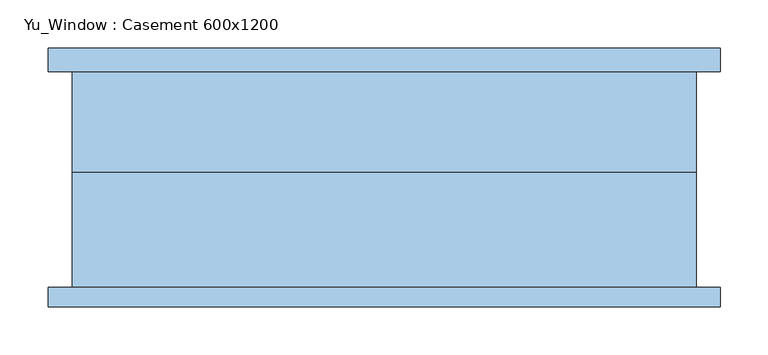
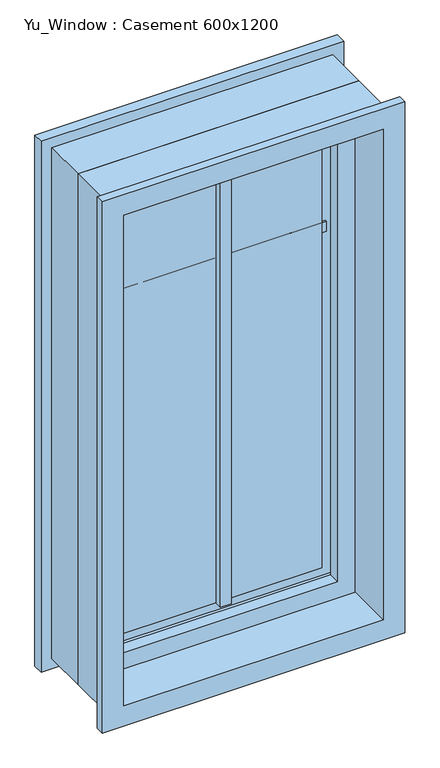
"""IFC4 building model written with IfcOpenShell, lengths in millimetres: window geometry, Yu_Window : Casement 600x1200."""

from ifc_helpers import new_model, si_unit, frame, origin, place, context, project, spatial, polyline, outline, extrude, faceted_brep, source, transform, mapped, element, save


def yu_window_casement_600x1200_84df8a12(model_context):
    return source(origin(), model_context, "Body", "SolidModel", [
        faceted_brep([(275.0, -12.5, 1775.0), (275.0, 7.5, 1775.0), (275.0, 7.5, 625.0), (275.0, -12.5, 625.0), (325.0, 7.5, 1825.0), (325.0, 7.5, 575.0), (-325.0, 7.5, 575.0), (-325.0, 7.5, 1825.0), (-275.0, 7.5, 1775.0), (-275.0, 7.5, 625.0), (-275.0, -12.5, 625.0), (-300.0, -12.5, 1800.0), (-300.0, -12.5, 600.0), (300.0, -12.5, 600.0), (300.0, -12.5, 1800.0), (-275.0, -12.5, 1775.0), (300.0, -132.5, 1800.0), (300.0, -132.5, 600.0), (-300.0, -132.5, 600.0), (-350.0, -132.5, 1850.0), (-350.0, -132.5, 550.0), (350.0, -132.5, 550.0), (350.0, -132.5, 1850.0), (-300.0, -132.5, 1800.0), (350.0, -112.5, 1850.0), (350.0, -112.5, 550.0), (-350.0, -112.5, 550.0), (-350.0, -112.5, 1850.0), (-325.0, -112.5, 1825.0), (-325.0, -112.5, 575.0), (325.0, -112.5, 575.0), (325.0, -112.5, 1825.0)], [[[0, 1, 2, 3]], [[4, 5, 6, 7], [8, 9, 2, 1]], [[3, 2, 9, 10]], [[11, 12, 13, 14], [0, 3, 10, 15]], [[16, 14, 13, 17]], [[17, 13, 12, 18]], [[19, 20, 21, 22], [16, 17, 18, 23]], [[24, 22, 21, 25]], [[25, 21, 20, 26]], [[24, 25, 26, 27], [28, 29, 30, 31]], [[4, 31, 30, 5]], [[5, 30, 29, 6]], [[10, 9, 8, 15]], [[18, 12, 11, 23]], [[26, 20, 19, 27]], [[6, 29, 28, 7]], [[15, 8, 1, 0]], [[23, 11, 14, 16]], [[27, 19, 22, 24]], [[7, 28, 31, 4]]]),
        faceted_brep([(-275.0, 32.5, 1775.0), (-275.0, 7.5, 1775.0), (-275.0, 7.5, 625.0), (-275.0, 32.5, 625.0), (-325.0, 7.5, 1825.0), (-325.0, 7.5, 575.0), (325.0, 7.5, 575.0), (325.0, 7.5, 1825.0), (275.0, 7.5, 1775.0), (275.0, 7.5, 625.0), (275.0, 32.5, 625.0), (300.0, 32.5, 1800.0), (300.0, 32.5, 600.0), (-300.0, 32.5, 600.0), (-300.0, 32.5, 1800.0), (275.0, 32.5, 1775.0), (-300.0, 137.5, 1800.0), (-300.0, 137.5, 600.0), (300.0, 137.5, 600.0), (350.0, 137.5, 1850.0), (350.0, 137.5, 550.0), (-350.0, 137.5, 550.0), (-350.0, 137.5, 1850.0), (300.0, 137.5, 1800.0), (-350.0, 112.5, 1850.0), (-350.0, 112.5, 550.0), (350.0, 112.5, 550.0), (350.0, 112.5, 1850.0), (325.0, 112.5, 1825.0), (325.0, 112.5, 575.0), (-325.0, 112.5, 575.0), (-325.0, 112.5, 1825.0)], [[[0, 1, 2, 3]], [[4, 5, 6, 7], [8, 9, 2, 1]], [[3, 2, 9, 10]], [[11, 12, 13, 14], [0, 3, 10, 15]], [[16, 14, 13, 17]], [[17, 13, 12, 18]], [[19, 20, 21, 22], [16, 17, 18, 23]], [[24, 22, 21, 25]], [[25, 21, 20, 26]], [[24, 25, 26, 27], [28, 29, 30, 31]], [[4, 31, 30, 5]], [[5, 30, 29, 6]], [[10, 9, 8, 15]], [[18, 12, 11, 23]], [[26, 20, 19, 27]], [[6, 29, 28, 7]], [[15, 8, 1, 0]], [[23, 11, 14, 16]], [[27, 19, 22, 24]], [[7, 28, 31, 4]]]),
        extrude(outline(polyline([(605.0, 295.0), (1795.0, 295.0), (1795.0, -295.0), (605.0, -295.0), (605.0, 295.0)]), holes=[polyline([(645.0, -255.0), (1755.0, -255.0), (1755.0, 255.0), (645.0, 255.0), (645.0, -255.0)])]), frame((0.0, -27.5, 0.0), z_axis=(0.0, 1.0, 0.0), x_axis=(0.0, 0.0, 1.0)), (0.0, 0.0, 1.0), 27.5),
        extrude(outline(polyline([(605.0, 295.0), (1795.0, 295.0), (1795.0, -295.0), (605.0, -295.0), (605.0, 295.0)]), holes=[polyline([(655.0, -245.0), (1745.0, -245.0), (1745.0, 245.0), (655.0, 245.0), (655.0, -245.0)])]), frame((0.0, 32.5, 0.0), z_axis=(0.0, 1.0, 0.0), x_axis=(0.0, 0.0, 1.0)), (0.0, 0.0, 1.0), 15.0),
        extrude(outline(polyline([(-245.0, 22.0), (245.0, 22.0), (245.0, 18.0), (-245.0, 18.0), (-245.0, 22.0)])), frame((0.0, 0.0, 655.0), z_axis=(0.0, 0.0, 1.0), x_axis=(1.0, 0.0, 0.0)), (0.0, 0.0, 1.0), 1090.0),
        extrude(outline(polyline([(25.0, 32.5), (25.0, 0.0), (0.0, 0.0), (0.0, 32.5), (25.0, 32.5)])), frame((0.0, 0.0, 655.0), z_axis=(0.0, 0.0, 1.0), x_axis=(1.0, 0.0, 0.0)), (0.0, 0.0, 1.0), 1140.0),
        extrude(outline(polyline([(-255.0, 18.0), (-255.0, 22.0), (255.0, 22.0), (255.0, 18.0), (-255.0, 18.0)])), frame((0.0, 0.0, 1475.0), z_axis=(0.0, 0.0, 1.0), x_axis=(1.0, 0.0, 0.0)), (0.0, 0.0, 1.0), 25.0),
    ])


if __name__ == "__main__":
    model = new_model("IFC4")
    model_context = context("Model", 3, world=origin())
    ifc_project = project(units=[si_unit("LENGTHUNIT", "METRE", prefix="MILLI")], contexts=[model_context])
    site = spatial("IfcSite", under=ifc_project)
    building = spatial("IfcBuilding", under=site)
    placement = place(None, origin())
    yu_window_casement_600x1200_shape = yu_window_casement_600x1200_84df8a12(model_context)
    element("IfcWindow", 1, ObjectType="Yu_Window : Casement 600x1200", at=placement, inside=building, context=model_context, shape_type="MappedRepresentation", body=[
        mapped(yu_window_casement_600x1200_shape, transform((0.0, 0.0, 0.0), x_axis=(1.0, 0.0, 0.0), y_axis=(0.0, 1.0, 0.0), z_axis=(0.0, 0.0, 1.0))),
    ])
    save(model, "model.ifc")

# Revit data of these elements
# Type "Yu_Window : Casement 600x1200"
#   Type Mark = "28"
#   Analytic Construction = "<None>"
#   mullion 2 = 300 mm
#   Window panel size 1 = 300 mm
#   Offset = 25 mm
#   Height = 1200 mm
#   Default Sill Height = 600 mm
#   Width = 600 mm
#   Define Thermal Properties by = 1
#   Interior material = none
#   Exterior material = none
#   Wall Closure = (empty or 0)
# Element 1 (IfcWindow, "Yu_Window : Casement 600x1200")
#   Materials on its faces: "Glass"
# Materials
#   "Glass": class "Glass", colour RGB 0 128 192, transparency 0.9, Description = "Soda Lime Glass", Cost = 0
